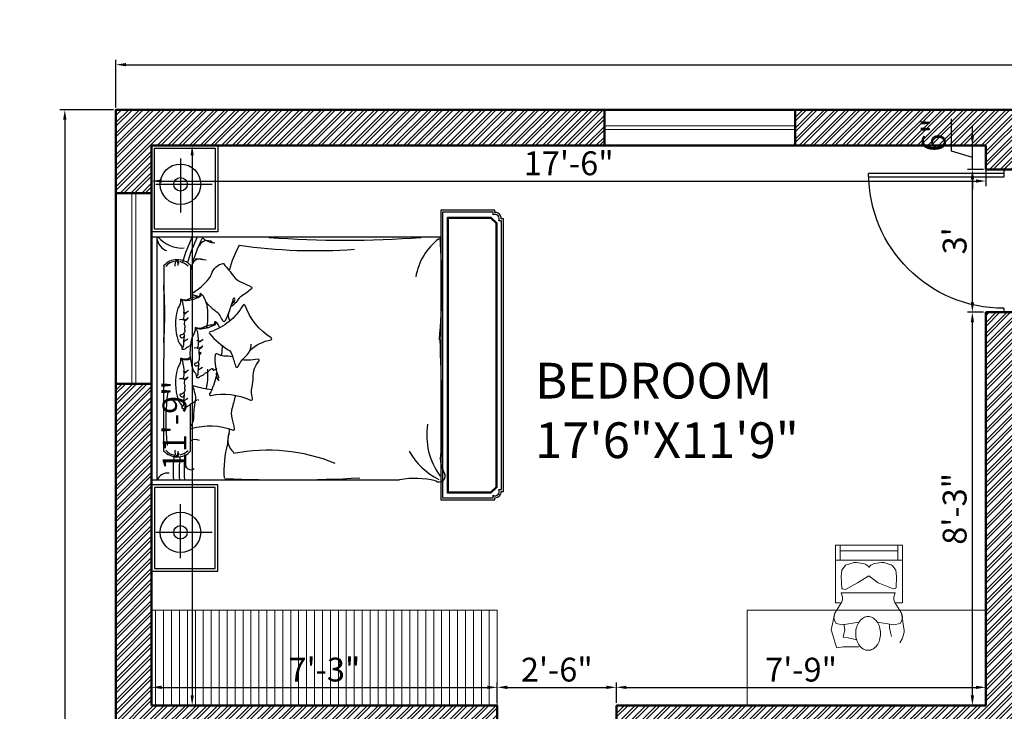
# Model space of a CAD drawing. Units: inches. Extents: x 3590 to 5167, y 65 to 1917.
# Tile 4 of 100: x 3621 to 3869, y 438 to 612. Entities that reach past the tile are written whole.
import ezdxf

# ---------------------------------------------------------------- set-up
doc = ezdxf.new("R2010")
doc.units = ezdxf.units.IN
for name, color, linetype, lineweight in [('A-ANNO-DIMS', 2, 'Continuous', 18), ('A-AREA-IDEN', 7, 'Continuous', 18), ('A-DOOR', 3, 'Continuous', 25), ('A-FURN', 21, 'Continuous', 18), ('A-GLAZ', 4, 'Continuous', 18), ('A-WALL', 7, 'Continuous', 50), ('A-WALL-PATT', 251, 'Continuous', 13)]:
    doc.layers.add(name, color=color, linetype=linetype, lineweight=lineweight)
for name, color, linetype in [('FUR', 42, 'Continuous'), ('HA-FUR', 8, 'Continuous'), ('HA-P', 8, 'Continuous'), ('SAN', 5, 'Continuous'), ('wood', 26, 'Continuous')]:
    doc.layers.add(name, color=color, linetype=linetype)
doc.styles.get("Standard").update_dxf_attribs({"font": 'arial.ttf'})
doc.dimstyles.new('ISO-25', dxfattribs={"dimtxt": 9, "dimasz": 2.5, "dimexe": 1.25, "dimexo": 0.625, "dimtad": 1, "dimdec": 1, "dimlunit": 3, "dimtxsty": 'Standard', "dimcen": 2.5, "dimadec": 0, "dimazin": 0, "dimtfac": 1, "dimtdec": 1, "dimtmove": 0, "dimatfit": 3, "dimfxl": 1, "dimarcsym": 0})

# ---------------------------------------------------------------- blocks, each defined once
blk = doc.blocks.new('*D247')
at = {"layer": 'A-ANNO-DIMS', "color": 0, "lineweight": -2, "transparency": 16777216}
for p, q in [((3645.51, 589.68), (3645.51, 601.68)), ((3648.01, 600.43), (4303.01, 600.43)), ((4305.51, 589.68), (4305.51, 601.68))]:
    blk.add_line(p, q, dxfattribs=at)
at = {"layer": 'A-ANNO-DIMS', "color": 0, "transparency": 16777216}
for points in [[(3648.01, 600.84), (3648.01, 600.01), (3645.51, 600.43)], [(4303.01, 600.84), (4303.01, 600.01), (4305.51, 600.43)]]:
    blk.add_solid(points, dxfattribs=at)
at = {"layer": 'Defpoints', "color": 0, "transparency": 16777216}
for p in [(4305.51, 600.43), (3645.51, 589.06), (4305.51, 589.06)]:
    blk.add_point(p, dxfattribs=at)
at = {"layer": 'A-ANNO-DIMS', "color": 0, "transparency": 16777216, "insert": (3975.51, 605.63), "char_height": 9, "attachment_point": 5}
blk.add_mtext("55'", dxfattribs=at)
blk = doc.blocks.new('*D248')
at = {"layer": 'A-ANNO-DIMS', "color": 0, "lineweight": -2, "transparency": 16777216}
for p, q in [((3644.89, 589.06), (3631.39, 589.06)), ((3632.64, 586.56), (3632.64, 111.56)), ((3644.89, 109.06), (3631.39, 109.06))]:
    blk.add_line(p, q, dxfattribs=at)
at = {"layer": 'A-ANNO-DIMS', "color": 0, "transparency": 16777216}
for points in [[(3632.22, 586.56), (3633.06, 586.56), (3632.64, 589.06)], [(3632.22, 111.56), (3633.06, 111.56), (3632.64, 109.06)]]:
    blk.add_solid(points, dxfattribs=at)
at = {"layer": 'Defpoints', "color": 0, "transparency": 16777216}
for p in [(3645.51, 589.06), (3632.64, 109.06), (3645.51, 109.06)]:
    blk.add_point(p, dxfattribs=at)
at = {"layer": 'A-ANNO-DIMS', "color": 0, "transparency": 16777216, "insert": (3627.42, 349.06), "char_height": 9, "attachment_point": 5, "rotation": 90}
blk.add_mtext("40'", dxfattribs=at)
blk = doc.blocks.new('D1')
for p, q in [((1, 0), (1, 34)), ((2, 0), (2, 33.99)), ((0, 0), (2, 0)), ((35, 0), (36, 0))]:
    blk.add_line(p, q)
at = {"ltscale": 0.5}
blk.add_arc((1, 0), 34, 0, 90, dxfattribs=at)
blk = doc.blocks.new('*D191')
at = {"layer": 'A-ANNO-DIMS', "color": 0, "lineweight": -2, "transparency": 16777216}
for p, q in [((3654.51, 579.43), (3654.51, 569.87)), ((3864.51, 579.43), (3864.51, 569.87)), ((3657.01, 571.12), (3862.01, 571.12))]:
    blk.add_line(p, q, dxfattribs=at)
at = {"layer": 'A-ANNO-DIMS', "color": 0, "transparency": 16777216}
for points in [[(3657.01, 571.54), (3657.01, 570.71), (3654.51, 571.12)], [(3862.01, 571.54), (3862.01, 570.71), (3864.51, 571.12)]]:
    blk.add_solid(points, dxfattribs=at)
at = {"layer": 'Defpoints', "color": 0, "transparency": 16777216}
for p in [(3654.51, 580.06), (3864.51, 580.06), (3864.51, 571.12)]:
    blk.add_point(p, dxfattribs=at)
at = {"layer": 'A-ANNO-DIMS', "color": 0, "transparency": 16777216, "insert": (3759.51, 574.81), "char_height": 6, "attachment_point": 5}
blk.add_mtext('17\'-6"', dxfattribs=at)
blk = doc.blocks.new('*D192')
at = {"layer": 'A-ANNO-DIMS', "color": 0, "lineweight": -2, "transparency": 16777216}
for p, q in [((3655.14, 580.06), (3665.95, 580.06)), ((3664.7, 577.56), (3664.7, 441.56)), ((3655.14, 439.06), (3665.95, 439.06))]:
    blk.add_line(p, q, dxfattribs=at)
at = {"layer": 'A-ANNO-DIMS', "color": 0, "transparency": 16777216}
for points in [[(3664.29, 577.56), (3665.12, 577.56), (3664.7, 580.06)], [(3664.29, 441.56), (3665.12, 441.56), (3664.7, 439.06)]]:
    blk.add_solid(points, dxfattribs=at)
at = {"layer": 'Defpoints', "color": 0, "transparency": 16777216}
for p in [(3654.51, 580.06), (3654.51, 439.06), (3664.7, 439.06)]:
    blk.add_point(p, dxfattribs=at)
at = {"layer": 'A-ANNO-DIMS', "color": 0, "transparency": 16777216, "insert": (3661.02, 509.56), "char_height": 6, "attachment_point": 5, "rotation": 90}
blk.add_mtext('11\'-9"', dxfattribs=at)
blk = doc.blocks.new('*D193')
at = {"layer": 'A-ANNO-DIMS', "color": 0, "lineweight": -2, "transparency": 16777216}
for p, q in [((3654.51, 439.68), (3654.51, 444.85)), ((3741.51, 439.68), (3741.51, 444.85)), ((3657.01, 443.6), (3739.01, 443.6))]:
    blk.add_line(p, q, dxfattribs=at)
at = {"layer": 'A-ANNO-DIMS', "color": 0, "transparency": 16777216}
for points in [[(3657.01, 444.01), (3657.01, 443.18), (3654.51, 443.6)], [(3739.01, 444.01), (3739.01, 443.18), (3741.51, 443.6)]]:
    blk.add_solid(points, dxfattribs=at)
at = {"layer": 'Defpoints', "color": 0, "transparency": 16777216}
for p in [(3741.51, 443.6), (3654.51, 439.06), (3741.51, 439.06)]:
    blk.add_point(p, dxfattribs=at)
at = {"layer": 'A-ANNO-DIMS', "color": 0, "transparency": 16777216, "insert": (3698.01, 447.29), "char_height": 6, "attachment_point": 5}
blk.add_mtext('7\'-3"', dxfattribs=at)
blk = doc.blocks.new('*D199')
at = {"layer": 'A-ANNO-DIMS', "color": 0, "lineweight": -2, "transparency": 16777216}
for p, q in [((3741.51, 439.68), (3741.51, 444.85)), ((3771.51, 439.68), (3771.51, 444.85)), ((3744.01, 443.6), (3769.01, 443.6))]:
    blk.add_line(p, q, dxfattribs=at)
at = {"layer": 'A-ANNO-DIMS', "color": 0, "transparency": 16777216}
for points in [[(3744.01, 444.01), (3744.01, 443.18), (3741.51, 443.6)], [(3769.01, 444.01), (3769.01, 443.18), (3771.51, 443.6)]]:
    blk.add_solid(points, dxfattribs=at)
at = {"layer": 'Defpoints', "color": 0, "transparency": 16777216}
for p in [(3771.51, 443.6), (3741.51, 439.06), (3771.51, 439.06)]:
    blk.add_point(p, dxfattribs=at)
at = {"layer": 'A-ANNO-DIMS', "color": 0, "transparency": 16777216, "insert": (3756.51, 447.28), "char_height": 6, "attachment_point": 5}
blk.add_mtext('2\'-6"', dxfattribs=at)
blk = doc.blocks.new('*D200')
at = {"layer": 'A-ANNO-DIMS', "color": 0, "lineweight": -2, "transparency": 16777216}
for p, q in [((3771.51, 439.68), (3771.51, 444.85)), ((3864.51, 439.68), (3864.51, 444.85)), ((3774.01, 443.6), (3862.01, 443.6))]:
    blk.add_line(p, q, dxfattribs=at)
at = {"layer": 'A-ANNO-DIMS', "color": 0, "transparency": 16777216}
for points in [[(3774.01, 444.01), (3774.01, 443.18), (3771.51, 443.6)], [(3862.01, 444.01), (3862.01, 443.18), (3864.51, 443.6)]]:
    blk.add_solid(points, dxfattribs=at)
at = {"layer": 'Defpoints', "color": 0, "transparency": 16777216}
for p in [(3864.51, 443.6), (3771.51, 439.06), (3864.51, 439.06)]:
    blk.add_point(p, dxfattribs=at)
at = {"layer": 'A-ANNO-DIMS', "color": 0, "transparency": 16777216, "insert": (3818.01, 447.28), "char_height": 6, "attachment_point": 5}
blk.add_mtext('7\'-9"', dxfattribs=at)
blk = doc.blocks.new('*D201')
at = {"layer": 'A-ANNO-DIMS', "color": 0, "lineweight": -2, "transparency": 16777216}
for p, q in [((3863.89, 538.06), (3859.88, 538.06)), ((3861.13, 441.56), (3861.13, 535.56)), ((3863.89, 439.06), (3859.88, 439.06))]:
    blk.add_line(p, q, dxfattribs=at)
at = {"layer": 'A-ANNO-DIMS', "color": 0, "transparency": 16777216}
for points in [[(3860.71, 535.56), (3861.55, 535.56), (3861.13, 538.06)], [(3860.71, 441.56), (3861.55, 441.56), (3861.13, 439.06)]]:
    blk.add_solid(points, dxfattribs=at)
at = {"layer": 'Defpoints', "color": 0, "transparency": 16777216}
for p in [(3861.13, 538.06), (3864.51, 538.06), (3864.51, 439.06)]:
    blk.add_point(p, dxfattribs=at)
at = {"layer": 'A-ANNO-DIMS', "color": 0, "transparency": 16777216, "insert": (3857.44, 488.56), "char_height": 6, "attachment_point": 5, "rotation": 90}
blk.add_mtext('8\'-3"', dxfattribs=at)
blk = doc.blocks.new('*D202')
at = {"layer": 'A-ANNO-DIMS', "color": 0, "lineweight": -2, "transparency": 16777216}
for p, q in [((3863.89, 574.06), (3859.88, 574.06)), ((3861.13, 540.56), (3861.13, 571.56)), ((3863.89, 538.06), (3859.88, 538.06))]:
    blk.add_line(p, q, dxfattribs=at)
at = {"layer": 'A-ANNO-DIMS', "color": 0, "transparency": 16777216}
for points in [[(3860.71, 571.56), (3861.55, 571.56), (3861.13, 574.06)], [(3860.71, 540.56), (3861.55, 540.56), (3861.13, 538.06)]]:
    blk.add_solid(points, dxfattribs=at)
at = {"layer": 'Defpoints', "color": 0, "transparency": 16777216}
for p in [(3861.13, 574.06), (3864.51, 574.06), (3864.51, 538.06)]:
    blk.add_point(p, dxfattribs=at)
at = {"layer": 'A-ANNO-DIMS', "color": 0, "transparency": 16777216, "insert": (3857.44, 556.06), "char_height": 6, "attachment_point": 5, "rotation": 90}
blk.add_mtext("3'", dxfattribs=at)
blk = doc.blocks.new('*D165')
at = {"layer": 'A-ANNO-DIMS', "color": 0, "lineweight": -2, "transparency": 16777216}
for p, q in [((3855.88, 578.64), (3855.88, 586.81)), ((3861.13, 582.56), (3861.13, 585.06)), ((3863.89, 580.06), (3859.88, 580.06)), ((3861.13, 574.06), (3861.13, 580.06)), ((3861.13, 574.06), (3861.13, 580.06)), ((3861.13, 577.06), (3855.88, 578.64)), ((3863.89, 574.06), (3859.88, 574.06)), ((3861.13, 571.56), (3861.13, 569.06))]:
    blk.add_line(p, q, dxfattribs=at)
at = {"layer": 'A-ANNO-DIMS', "color": 0, "transparency": 16777216}
for points in [[(3860.71, 582.56), (3861.55, 582.56), (3861.13, 580.06)], [(3860.71, 571.56), (3861.55, 571.56), (3861.13, 574.06)]]:
    blk.add_solid(points, dxfattribs=at)
at = {"layer": 'Defpoints', "color": 0, "transparency": 16777216}
for p in [(3861.13, 580.06), (3864.51, 580.06), (3864.51, 574.06)]:
    blk.add_point(p, dxfattribs=at)
at = {"layer": 'A-ANNO-DIMS', "color": 0, "transparency": 16777216, "insert": (3852.19, 582.72), "char_height": 6, "attachment_point": 5, "rotation": 90}
blk.add_mtext('6"', dxfattribs=at)
blk = doc.blocks.new('A$C0A42580C')
at = {"layer": 'SAN'}
for p, q in [((0.2873, 0.0301), (0.2873, 0.4484)), ((2.8678, 0.0301), (2.8678, 0.4484)), ((0.0949, 0.2135), (0.4958, 0.2135)), ((3.0601, 0.2135), (2.6592, 0.2135))]:
    blk.add_line(p, q, dxfattribs=at)
for centre, radius in [((0.2873, 0.2135), 0.15), ((2.8678, 0.2135), 0.15), ((0.2873, 0.2135), 0.05), ((2.8678, 0.2135), 0.05)]:
    blk.add_circle(centre, radius, dxfattribs=at)
at = {"layer": 'wood'}
for p, q in [((0.6775, 0.8851), (0.6775, 2.1392)), ((2.4775, 0.8016), (2.4775, 1.838)), ((2.4775, 0), (2.4775, 0.8016)), ((1.6633, 0.3438), (1.6434, 0.3761)), ((1.5, 0.3423), (1.5016, 0.3142)), ((0.888, 0.289), (1.1327, 0.289)), ((1.2906, 0.2348), (1.2921, 0.2067)), ((1.4538, 0.2362), (1.434, 0.2685)), ((1.7287, 0.2348), (1.7302, 0.2067)), ((1.8919, 0.2362), (1.8721, 0.2685)), ((2.267, 0.289), (1.9163, 0.289)), ((0.8909, 0.089), (1.5775, 0.089)), ((2.2642, 0.089), (1.5775, 0.089)), ((0.6775, 0.039), (2.4775, 0.039)), ((0.6775, 0), (2.4775, 0))]:
    blk.add_line(p, q, dxfattribs=at)
blk.add_lwpolyline([(0.6775, 0), (0.6775, 0.8851)], dxfattribs=at)
for points in [[(1.516, 0.7294, -0.128392), (1.4401, 0.8834, 0.70791), (1.427, 0.8863, -0.16964), (1.1848, 0.6919, 0.664036), (1.184, 0.6776, -0.184649), (1.3819, 0.4332, 0.662242), (1.3969, 0.4309, 0.078539), (1.5137, 0.5669, -0.1736), (1.5484, 0.5947, -0.02159), (1.6357, 0.6205, 0.697276), (1.6379, 0.6405, -0.093019), (1.5606, 0.699, 0.216632), (1.4719, 0.7371, -2.511293)], [(1.1211, 0.3454, 0.032543), (1.1095, 0.3091, -0.658965), (1.0917, 0.3063, 0.074753), (0.9887, 0.4234, 0.100988), (0.953, 0.4429, -0.270711), (0.8753, 0.5273, -0.276825), (0.8775, 0.5337, -0.014937), (0.9701, 0.6081, 0.134834), (1.0135, 0.6643, -0.023706), (1.0474, 0.7372, -0.664036), (1.0616, 0.7394, -0.035987), (1.119, 0.6627, 0.118631), (1.1415, 0.6412, -0.132738), (1.1955, 0.5864)], [(1.6795, 0.4818, 0.263265), (1.7191, 0.4839, -0.026108), (1.743, 0.4973, 0.027613), (1.7137, 0.4764, -0.089259), (1.8403, 0.429, 0.662242), (1.8528, 0.4376, -0.162037), (1.8882, 0.732, 0.676499), (1.8733, 0.748, -0.160513), (1.7901, 0.7439, 0.07473), (1.7202, 0.7523, -0.187721), (1.5966, 0.7963, 0.70791), (1.5851, 0.7895, -0.010003), (1.5921, 0.7143, -0.07079), (1.5891, 0.6719, 0.099539)], [(1.1759, 0.5928, 0.013884), (1.1549, 0.6131, 0.174178), (1.1437, 0.6177, 0.104076), (1.1358, 0.6165, 0.389829), (1.1324, 0.6097, 0.296089), (1.1415, 0.6019, -0.036701), (1.1572, 0.5985, -0.040547), (1.3022, 0.543, -0.70791), (1.3021, 0.5296, -0.016811), (1.2631, 0.5085, 0.11866), (1.2414, 0.4904, -0.048791), (1.1649, 0.4055, 0.103757)], [(1.5674, 0.601, 0.057807), (1.5606, 0.5339, -0.173425), (1.5457, 0.49, 0.589988), (1.5538, 0.4706, 0.137312), (1.7236, 0.4985, 0.137312)], [(1.8113, 0.4446, -0.069098), (1.7831, 0.3187, 0.658965), (1.7961, 0.3062, -0.049789), (1.8516, 0.3234, -0.103757), (1.8905, 0.3233, 0.055725), (2.0203, 0.3103, -0.11866), (2.0478, 0.304, 0.016811), (2.0881, 0.2856, 0.70791), (2.0989, 0.2936, -0.16964), (2.1104, 0.604, 0.664036), (2.1001, 0.6139, 0.023706), (2.0214, 0.597, -0.134834), (1.9505, 0.5976, 0.012748), (1.8522, 0.6228)], [(1.3107, 0.4764, 0.145733), (1.3069, 0.4677, 0.488583), (1.3089, 0.4657, -0.012138), (1.3131, 0.4661, -0.125673), (1.3213, 0.4646, -0.750706)], [(1.3153, 0.4751, -0.274893), (1.3379, 0.4529, 0.051436), (1.3468, 0.4293, -0.086628), (1.3532, 0.4078, 0.040196), (1.3593, 0.3772, -0.184744), (1.3556, 0.3344, -2.554464)], [(1.317, 0.4683, -0.060098), (1.3283, 0.4571, -0.16247), (1.3313, 0.4487, 0.120018), (1.3493, 0.3815, -0.060072), (1.3541, 0.3695, -0.13107), (1.3541, 0.3395, -0.024415), (1.3534, 0.3373, 0.070398), (1.3503, 0.3233, 0.528689), (1.3524, 0.3216, -0.069388), (1.3557, 0.3222, -0.158233), (1.4075, 0.3065, 0.085461), (1.4255, 0.2981, 0.147196), (1.6571, 0.3041, 0.10985), (1.6823, 0.3191, -0.179095), (1.7126, 0.3319, -2.318897)], [(1.1013, 0.3688, 0.145733), (1.0975, 0.3601, 0.488583), (1.0995, 0.3581, -0.012138), (1.1036, 0.3585, -0.125673), (1.1119, 0.357, -0.750706)], [(1.1059, 0.3675, -0.274893), (1.1285, 0.3453, 0.051436), (1.1373, 0.3217, -0.086628), (1.1438, 0.3003, 0.040196), (1.1499, 0.2696, -0.184744), (1.1462, 0.2269, -2.554464)], [(1.4359, 0.3803, -0.198519), (1.452, 0.3494, 0.826402), (1.4558, 0.349, 0.095956), (1.4561, 0.3528, 0.242899), (1.4461, 0.3686, -17.523452)], [(1.5447, 0.3525, -0.083557), (1.507, 0.3546, 0.203162), (1.4851, 0.3792, -0.208037), (1.5043, 0.3409, 0.124669), (1.4432, 0.3469, 0.965934)], [(1.5394, 0.3688, 0.145733), (1.5356, 0.3601, 0.488583), (1.5376, 0.3581, -0.012138), (1.5418, 0.3585, -0.125673), (1.55, 0.357, -0.750706)], [(1.1076, 0.3607, -0.060098), (1.1189, 0.3495, -0.16247), (1.1219, 0.3411, 0.120018), (1.1399, 0.2739, -0.060072), (1.1447, 0.2619, -0.13107), (1.1447, 0.2319, -0.024415), (1.144, 0.2297, 0.070398), (1.1409, 0.2157, 0.528689), (1.143, 0.2141, -0.069388), (1.1463, 0.2146, -0.158233), (1.1981, 0.1989, 0.085461), (1.2161, 0.1905, 0.147196), (1.4477, 0.1965, 0.10985), (1.4728, 0.2115, -0.179095), (1.5032, 0.2244, -2.318897)], [(1.3509, 0.3219, -0.117141), (1.3688, 0.335, -0.025084), (1.4533, 0.348, 0.033691)], [(1.5447, 0.3525, -0.008229), (1.5728, 0.3519, 0.033691)], [(1.5728, 0.3519, -0.46905), (1.6152, 0.321, 0.420988), (1.62, 0.3169, 0.857652), (1.6221, 0.3484, 0.548526)], [(1.603, 0.3451, -0.099719), (1.6221, 0.3484, 0.102691)], [(1.6214, 0.3487, -0.010168), (1.6558, 0.3447, 0.033691), (1.6907, 0.3423, -0.220869), (1.7148, 0.3311, -0.288972)], [(1.1415, 0.2143, -0.117141), (1.1594, 0.2274, -0.025084), (1.2439, 0.2405, 0.033691)], [(1.2265, 0.2728, -0.198519), (1.2426, 0.2418, 0.826402), (1.2463, 0.2415, 0.095956), (1.2467, 0.2452, 0.242899), (1.2366, 0.2611, -17.523452)], [(1.3353, 0.2449, -0.083557), (1.2976, 0.247, 0.203162), (1.2757, 0.2717, -0.208037), (1.2948, 0.2333, 0.124669), (1.2338, 0.2393, 0.965934)], [(1.3353, 0.2449, -0.008229), (1.3633, 0.2443, 0.033691)], [(1.3633, 0.2443, -0.46905), (1.4058, 0.2134, 0.420988), (1.4106, 0.2093, 0.857652), (1.4127, 0.2408, 0.548526)], [(1.3936, 0.2375, -0.099719), (1.4127, 0.2408, 0.102691)], [(1.412, 0.2411, -0.010168), (1.4464, 0.2371, 0.033691), (1.4812, 0.2348, -0.220869), (1.5054, 0.2235, -0.288972)], [(1.5721, 0.286, 0.022869), (1.578, 0.2739, -0.060072), (1.5828, 0.2619, -0.13107), (1.5828, 0.2319, -0.024415), (1.5821, 0.2297, 0.070398), (1.579, 0.2157, 0.528689), (1.5811, 0.2141, -0.069388), (1.5844, 0.2146, -0.158233), (1.6362, 0.1989, 0.085461), (1.6542, 0.1905, 0.147196), (1.8858, 0.1965, 0.10985), (1.911, 0.2115, -0.179095), (1.9413, 0.2244, -2.318897)], [(1.5796, 0.2143, -0.117141), (1.5975, 0.2274, -0.025084), (1.682, 0.2405, 0.033691)], [(1.5838, 0.2873, 0.023398), (1.588, 0.2696, -0.184744), (1.5843, 0.2269, -2.554464)], [(1.6646, 0.2728, -0.198519), (1.6807, 0.2418, 0.826402), (1.6845, 0.2415, 0.095956), (1.6848, 0.2452, 0.242899), (1.6748, 0.2611, -17.523452)], [(1.7734, 0.2449, -0.083557), (1.7357, 0.247, 0.203162), (1.7138, 0.2717, -0.208037), (1.733, 0.2333, 0.124669), (1.6719, 0.2393, 0.965934)], [(1.7734, 0.2449, -0.008229), (1.8015, 0.2443, 0.033691)], [(1.8015, 0.2443, -0.46905), (1.8439, 0.2134, 0.420988), (1.8487, 0.2093, 0.857652), (1.8508, 0.2408, 0.548526)], [(1.8317, 0.2375, -0.099719), (1.8508, 0.2408, 0.102691)], [(1.8501, 0.2411, -0.010168), (1.8845, 0.2371, 0.033691), (1.9193, 0.2348, -0.220869), (1.9435, 0.2235, -0.288972)]]:
    blk.add_lwpolyline(points, format="xyb", dxfattribs=at)
for points in [[(0.64, 0), (0, 0), (0, 0.49), (0.64, 0.49)], [(0.62, 0.02), (0.02, 0.02), (0.02, 0.47), (0.62, 0.47)], [(2.515, 0), (3.155, 0), (3.155, 0.49), (2.515, 0.49)], [(2.535, 0.02), (3.135, 0.02), (3.135, 0.47), (2.535, 0.47)]]:
    blk.add_lwpolyline(points, close=True, dxfattribs=at)
for centre, radius, start, end in [((1.0344, -2.14), 4.292, 84.56078, 94.7164), ((1.0494, 2.4026), 0.4515, 217.47941, 260.35986), ((2.0208, -11.0786), 13.2288, 88.75549, 92.51133), ((2.1491, 2.5471), 0.5083, 260.65485, 306.44155), ((2.3125, 2.3833), 0.2443, 254.1515, 300.95574), ((2.0168, 2.3573), 0.5127, 299.08175, 333.44367), ((2.4501, 2.1309), 0.0445, 324.18954, 118.92203), ((3.1371, 1.9502), 0.669, 166.6404, 189.65708), ((-7.0839, 1.4328), 7.7858, 355.84817, 4.15183), ((-7.2439, 0.9937), 9.7233, 357.34474, 3.23068), ((-3.167, 1.2143), 3.9465, 351.77286, 4.18386), ((3.5803, 0.8622), 1.3213, 157.81295, 191.15154), ((1.1611, 1.4181), 0.8768, 241.21362, 254.41879), ((2.181, 0.6859), 0.1221, 247.37754, 321.13165), ((1.2583, 0.6364), 0.0695, 238.58923, 301.92671), ((1.4714, 0.0722), 0.4528, 80.62397, 88.74059), ((1.4035, -0.3388), 0.8693, 79.71489, 80.62397), ((1.7861, -2.1601), 2.7557, 80.89877, 83.46656), ((2.4192, 1.3819), 0.8461, 255.77539, 273.25587), ((0.5904, 0.4689), 0.13, 317.38218, 359.70393), ((0.7723, 0.4131), 0.0674, 147.68233, 245.79865), ((1.3546, 0.4469), 0.0529, 114.21284, 146.15395), ((2.6126, -2.3504), 3.1201, 113.83178, 114.21284), ((1.6301, 0.4539), 0.0342, 31.14095, 54.95422), ((1.6709, 0.4489), 0.0156, 131.9623, 212.08127), ((1.6729, 0.4422), 0.0178, 140.41793, 157.63267), ((1.7235, 0.4818), 0.0777, 212.08127, 227.364), ((1.6635, 0.4499), 0.00568, 95.52245, 140.41793), ((1.5664, 0.4154), 0.1086, 24.20989, 31.14095), ((1.6627, 0.4587), 0.00309, 275.52245, 24.20989), ((1.1611, 1.3191), 1.0568, 242.76671, 257.10398), ((0.0312, 0.4583), 0.8174, 350.42368, 356.2506), ((0.9021, 0.3562), 0.0605, 155.8342, 254.41058), ((1.1452, 0.3394), 0.0529, 114.21284, 146.15395), ((2.4032, -2.458), 3.1201, 113.55686, 114.21284), ((1.2046, 0.2912), 0.121, 99.42032, 113.55686), ((1.2774, -0.1478), 0.5659, 95.90379, 99.42032), ((1.2626, -0.005), 0.4223, 88.74059, 95.90379), ((1.2619, -0.0354), 0.4528, 80.62397, 88.74059), ((1.1941, -0.4464), 0.8693, 79.45871, 80.62397), ((1.4207, 0.3463), 0.0342, 31.14095, 54.95422), ((1.7007, -0.005), 0.4223, 88.74059, 95.90379), ((1.6391, 0.3902), 0.0469, 17.32618, 47.364), ((1.7106, 0.4125), 0.028, 197.32618, 226.17302), ((1.6431, 0.3422), 0.0695, 26.61764, 46.17302), ((1.8202, 0.431), 0.1287, 206.61764, 215.96192), ((1.7001, -0.0354), 0.4528, 80.62397, 88.74059), ((1.6322, -0.4464), 0.8693, 78.43923, 80.62397), ((1.1611, 1.3191), 1.0937, 243.75553, 254.4906), ((1.1611, 1.2816), 1.0937, 243.75553, 254.38927), ((1.4614, 0.3413), 0.0156, 131.9623, 212.08127), ((1.4635, 0.3347), 0.0178, 140.41793, 157.63267), ((1.4541, 0.3424), 0.00568, 95.52245, 140.41793), ((1.357, 0.3078), 0.1086, 24.20989, 31.14095), ((1.4533, 0.3511), 0.00309, 275.52245, 24.20989), ((1.5012, 0.305), 0.028, 197.32618, 226.17302), ((1.715, 0.3349), 0.00379, 207.1817, 328.02977), ((1.6975, 0.3419), 0.023, 350.76434, 35.96192), ((1.7058, 0.3406), 0.0145, 328.02977, 350.76434), ((1.9016, 0.3347), 0.0178, 140.41793, 157.63267), ((1.9522, 0.3743), 0.0777, 212.08127, 227.364), ((1.8922, 0.3424), 0.00568, 95.52245, 140.41793), ((1.8678, 0.2827), 0.0469, 17.32618, 47.364), ((1.9393, 0.305), 0.028, 197.32618, 226.17302), ((2.2511, 0.3256), 0.071, 155.86842, 211.04513), ((2.3616, 0.2915), 0.0419, 290.78583, 35.36309), ((0.5293, 0.2241), 0.2307, 309.63048, 4.27465), ((0.9846, 0.1903), 0.1381, 134.39284, 227.23745), ((0.9986, 0.1735), 0.1427, 136.58239, 164.9725), ((1.4337, 0.2347), 0.0695, 26.61764, 46.17302), ((1.6108, 0.3235), 0.1287, 206.61764, 215.96192), ((1.5055, 0.2273), 0.00379, 207.1817, 328.02977), ((1.4881, 0.2344), 0.023, 350.76434, 35.96192), ((1.4964, 0.233), 0.0145, 328.02977, 350.76434), ((1.8718, 0.2347), 0.0695, 26.61764, 46.17302), ((2.0489, 0.3235), 0.1287, 206.61764, 215.96192), ((1.9436, 0.2273), 0.00379, 207.1817, 328.02977), ((1.9262, 0.2344), 0.023, 350.76434, 35.96192), ((1.9345, 0.233), 0.0145, 328.02977, 350.76434), ((2.1565, 0.1735), 0.1427, 15.0275, 43.41761), ((2.1704, 0.1903), 0.1381, 312.76255, 45.60716), ((2.4192, 1.2667), 1.0261, 263.09035, 273.25587), ((0.8396, 0.185), 0.0112, 314.89662, 45.10338), ((0.8413, 0.1846), 0.0128, 299.47062, 57.44416), ((0.8844, 0.2286), 0.0569, 229.70587, 281.11527), ((0.8802, 0.1371), 0.0592, 81.47786, 123.11925), ((0.8698, 0.1793), 0.0229, 77.14902, 159.1786), ((0.9466, 0.1765), 0.0862, 185.53723, 234.68694), ((2.2085, 0.1765), 0.0862, 305.31306, 354.46277), ((2.2706, 0.2286), 0.0569, 258.88473, 310.29413), ((2.2749, 0.1371), 0.0592, 56.88075, 98.52214), ((2.2853, 0.1793), 0.0229, 20.8214, 102.85098), ((2.4192, 1.2218), 1.0629, 263.23622, 273.25587), ((2.3138, 0.1846), 0.0128, 122.55584, 240.52938), ((2.3154, 0.185), 0.0112, 134.89662, 225.10338), ((2.4192, 1.2667), 1.0629, 263.94374, 273.25587), ((0.6729, 0.151), 0.1135, 279.23824, 338.73819), ((1.2481, -2.5919), 2.6893, 85.4722, 94.5278), ((2.0447, 1.7022), 1.5979, 262.13639, 276.48786), ((2.508, 0.1152), 0.0792, 169.94668, 248.24015)]:
    blk.add_arc(centre, radius, start, end, dxfattribs=at)
blk = doc.blocks.new('A$C623F1DA0')
at = {"layer": 'FUR'}
blk.add_lwpolyline([(0.628, 2.912, 0.414214), (0.562, 2.978), (0.562, 3), (0, 3), (0, 0), (0.562, 0), (0.562, 0.022, 0.414214), (0.628, 0.088), (0.65, 0.088), (0.65, 2.912)], format="xyb", close=True, dxfattribs=at)
at = {"layer": 'HA-FUR'}
blk.add_lwpolyline([(0.603, 2.892, 0.710288), (0.542, 2.953), (0.542, 2.98), (0.02, 2.98), (0.02, 0.02), (0.542, 0.02), (0.542, 0.047, 0.710288), (0.603, 0.108), (0.63, 0.108), (0.63, 2.892)], format="xyb", close=True, dxfattribs=at)
at = {"layer": 'HA-P'}
for points in [[(0.07, 2.93), (0.521, 2.93), (0.58, 2.871), (0.58, 0.129), (0.521, 0.07), (0.07, 0.07)], [(0.08, 2.92), (0.517, 2.92), (0.57, 2.867), (0.57, 0.133), (0.517, 0.08), (0.08, 0.08)]]:
    blk.add_lwpolyline(points, close=True, dxfattribs=at)

msp = doc.modelspace()

# ---------------------------------------------------------------- hatches: boundary and pattern name
at = {"layer": 'A-WALL-PATT', "transparency": 33554687}
h = msp.add_hatch(dxfattribs=at)
h.set_pattern_fill('ANSI32', color=256, scale=0.2)
h.set_pattern_definition([(45, (0, -1216.9392), (-1.3470384, 1.3470384), []), (45, (0.898, -1216.9392), (-1.3470384, 1.3470384), [])])
h.paths.add_polyline_path([(3768.51, 589.06), (3645.51, 589.06), (3645.51, 568.06), (3654.51, 568.06), (3654.51, 580.06), (3671.16, 580.06), (3768.51, 580.06)])
h.paths.add_polyline_path([(3909.51, 589.06), (3816.51, 589.06), (3816.51, 580.06), (3864.51, 580.06), (3864.51, 574.06), (3873.51, 574.06), (3873.51, 580.06), (3909.51, 580.06)])
h.paths.add_polyline_path([(4053.51, 589.06), (3969.51, 589.06), (3969.51, 580.06), (4053.51, 580.06)])
h.paths.add_polyline_path([(4215.51, 589.06), (4113.51, 589.06), (4113.51, 580.06), (4206.51, 580.06), (4206.51, 574.06), (4215.51, 574.06)])
h.paths.add_polyline_path([(3654.51, 520.06), (3645.51, 520.06), (3645.51, 403.06), (3654.51, 403.06), (3654.51, 433.06), (3741.51, 433.06), (3741.51, 439.06), (3654.51, 439.06)], flags=17)
h.paths.add_polyline_path([(3873.51, 538.06), (3864.51, 538.06), (3864.51, 439.06), (3771.51, 439.06), (3771.51, 433.06), (3774.51, 433.06), (3774.51, 337.06), (3654.51, 337.06), (3654.51, 367.06), (3645.51, 367.06), (3645.51, 322.06), (3654.51, 322.06), (3654.51, 328.06), (3864.51, 328.06), (3864.51, 322.06), (3873.51, 322.06), (3873.51, 367.06), (3864.51, 367.06), (3864.51, 337.06), (3780.51, 337.06), (3780.51, 433.06), (3864.51, 433.06), (3864.51, 403.06), (3873.51, 403.06)])
h.paths.add_polyline_path([(3654.51, 274.06), (3645.51, 274.06), (3645.51, 109.06), (3810.51, 109.06), (3810.51, 118.06), (3809.96, 118.06), (3654.51, 118.06)])
h.paths.add_polyline_path([(3915.51, 118.06), (3873.51, 118.06), (3873.51, 135.93), (3873.51, 205.06), (3876.51, 205.06), (3876.51, 214.06), (3864.51, 214.06), (3864.51, 118.06), (3858.51, 118.06), (3858.51, 109.06), (3915.51, 109.06)])
h.paths.add_polyline_path([(4028.01, 118.06), (4002.51, 118.06), (4002.51, 286.06), (3981.51, 286.06), (3981.51, 277.06), (3993.51, 277.06), (3993.51, 214.06), (3921.51, 214.06), (3921.51, 277.06), (3933.51, 277.06), (3933.51, 286.06), (3864.51, 286.06), (3864.51, 277.06), (3912.51, 277.06), (3912.51, 214.06), (3906.51, 214.06), (3906.51, 205.06), (3993.51, 205.06), (3993.51, 118.06), (3951.51, 118.06), (3951.51, 109.06), (4028.01, 109.06)])
h.paths.add_polyline_path([(4203.51, 118.06), (4158.51, 118.06), (4158.51, 310.06), (4194.51, 310.06), (4194.51, 319.06), (4149.51, 319.06), (4149.51, 118.06), (4124.01, 118.06), (4124.01, 109.06), (4203.51, 109.06)])
h.paths.add_polyline_path([(4305.51, 349.06), (4296.51, 349.06), (4296.51, 319.06), (4278.64, 319.06), (4260.51, 319.06), (4260.51, 310.06), (4296.51, 310.06), (4296.51, 304.06), (4305.51, 304.06)])
h.paths.add_polyline_path([(4305.51, 256.06), (4296.51, 256.06), (4296.51, 118.06), (4251.51, 118.06), (4251.51, 109.06), (4305.51, 109.06)])
h.paths.add_polyline_path([(4305.51, 460.06), (4215.51, 460.06), (4215.51, 526.06), (4206.51, 526.06), (4206.51, 460.06), (4149.51, 460.06), (4149.51, 451.06), (4296.51, 451.06), (4296.51, 421.06), (4305.51, 421.06)])

# ---------------------------------------------------------------- linework, layer by layer
at = {"layer": 'A-FURN'}
for p, q in [((3826.65, 479.38), (3826.65, 464.87)), ((3843.5, 479.38), (3826.65, 479.38)), ((3827.81, 475.61), (3827.81, 479.38)), ((3842.4, 475.61), (3842.4, 479.38)), ((3843.5, 464.87), (3843.5, 479.38)), ((3842.4, 477.94), (3827.81, 477.94)), ((3843.5, 475.61), (3826.65, 475.61)), ((3828.27, 473.11), (3829.16, 474.36)), ((3829.16, 474.36), (3831.09, 474.95)), ((3831.91, 475.02), (3833.56, 474.82)), ((3834.86, 474.09), (3835.08, 473.82)), ((3835.29, 474.09), (3835.08, 473.82)), ((3838.24, 475.02), (3836.59, 474.82)), ((3840.35, 474.56), (3839.07, 474.95)), ((3841.88, 473.11), (3841.38, 473.82)), ((3828.09, 471.5), (3828.27, 473.11)), ((3828.26, 468.51), (3828.09, 471.5)), ((3835.08, 471.68), (3832.21, 469.88)), ((3837.4, 469.88), (3835.08, 471.68)), ((3842.06, 471.5), (3841.88, 473.11)), ((3841.9, 468.66), (3842.06, 471.5)), ((3832.21, 469.88), (3829.16, 468.27)), ((3841.17, 468.45), (3837.4, 469.88)), ((3841.83, 468.58), (3841.17, 468.45)), ((3828.09, 467.38), (3841.7, 467.38)), ((3841.7, 467.38), (3828.09, 467.38)), ((3828.09, 467.38), (3828.34, 466.63)), ((3829.16, 468.27), (3828.33, 468.44)), ((3841.7, 467.38), (3841.46, 466.63)), ((3828.16, 464.98), (3826.53, 462.27)), ((3826.65, 464.87), (3828.09, 464.87)), ((3841.64, 464.98), (3843.26, 462.27)), ((3841.7, 464.87), (3843.5, 464.87)), ((3654.51, 463.06), (3741.51, 463.06)), ((3655.51, 463.06), (3655.51, 439.06)), ((3657.51, 463.06), (3657.51, 439.06)), ((3659.51, 463.06), (3659.51, 439.06)), ((3661.51, 463.06), (3661.51, 439.06)), ((3663.51, 463.06), (3663.51, 439.06)), ((3665.51, 463.06), (3665.51, 439.06)), ((3667.51, 463.06), (3667.51, 439.06)), ((3669.51, 463.06), (3669.51, 439.06)), ((3671.51, 463.06), (3671.51, 439.06)), ((3673.51, 463.06), (3673.51, 439.06)), ((3675.51, 463.06), (3675.51, 439.06)), ((3677.51, 463.06), (3677.51, 439.06)), ((3679.51, 463.06), (3679.51, 439.06)), ((3681.51, 463.06), (3681.51, 439.06)), ((3683.51, 463.06), (3683.51, 439.06)), ((3685.51, 463.06), (3685.51, 439.06)), ((3687.51, 463.06), (3687.51, 439.06)), ((3689.51, 463.06), (3689.51, 439.06)), ((3691.51, 463.06), (3691.51, 439.06)), ((3693.51, 463.06), (3693.51, 439.06)), ((3695.51, 463.06), (3695.51, 439.06)), ((3697.51, 463.06), (3697.51, 439.06)), ((3699.51, 463.06), (3699.51, 439.06)), ((3701.51, 463.06), (3701.51, 439.06)), ((3703.51, 463.06), (3703.51, 439.06)), ((3705.51, 463.06), (3705.51, 439.06)), ((3707.51, 463.06), (3707.51, 439.06)), ((3709.51, 463.06), (3709.51, 439.06)), ((3711.51, 463.06), (3711.51, 439.06)), ((3713.51, 463.06), (3713.51, 439.06)), ((3715.51, 463.06), (3715.51, 439.06)), ((3717.51, 463.06), (3717.51, 439.06)), ((3719.51, 463.06), (3719.51, 439.06)), ((3721.51, 463.06), (3721.51, 439.06)), ((3723.51, 463.06), (3723.51, 439.06)), ((3725.51, 463.06), (3725.51, 439.06)), ((3727.51, 463.06), (3727.51, 439.06)), ((3729.51, 463.06), (3729.51, 439.06)), ((3731.51, 463.06), (3731.51, 439.06)), ((3733.51, 463.06), (3733.51, 439.06)), ((3735.51, 463.06), (3735.51, 439.06)), ((3737.51, 463.06), (3737.51, 439.06)), ((3739.51, 463.06), (3739.51, 439.06)), ((3741.51, 463.06), (3741.51, 439.06)), ((3804.47, 463.06), (3864.51, 463.06)), ((3804.47, 463.06), (3804.47, 439.06)), ((3843.26, 462.27), (3843.92, 457.92)), ((3826.5, 460.29), (3826.83, 459.68)), ((3826.83, 459.68), (3828.45, 459.32)), ((3828.45, 459.32), (3832.57, 460.04)), ((3841.35, 459.32), (3837.23, 460.04)), ((3842.96, 459.68), (3841.35, 459.32)), ((3843.3, 460.29), (3842.96, 459.68))]:
    msp.add_line(p, q, dxfattribs=at)
for points in [[(3826.53, 462.27), (3825.58, 458.07), (3826.12, 456.45), (3826.65, 454.48), (3827.01, 453.59), (3828.63, 453.77), (3830.24, 453.77), (3832.57, 453.77)], [(3832.03, 455.56), (3829.88, 456.1), (3828.63, 456.27), (3828.98, 458.07), (3828.8, 459.5)], [(3840.77, 456.44), (3840.55, 457.38), (3840.3, 458.61), (3840.3, 459.49)], [(3842.83, 454.84), (3843.48, 455.82), (3843.77, 456.8), (3843.92, 457.58), (3843.92, 458.02)]]:
    msp.add_lwpolyline(points, dxfattribs=at)
msp.add_lwpolyline([(3838.01, 457.17, 0.07405), (3837.76, 458.85, 0.084801), (3837.09, 460.17, 0.106336), (3836.03, 461.12, 0.128955), (3834.88, 461.42, 0.128955), (3833.74, 461.12, 0.106336), (3832.68, 460.17, 0.084801), (3832.01, 458.85, 0.07405), (3831.76, 457.17, 0.07405), (3832.01, 455.49, 0.084801), (3832.68, 454.17, 0.106336), (3833.74, 453.22, 0.128955), (3834.88, 452.92, 0.128955), (3836.03, 453.22, 0.106336), (3837.09, 454.17, 0.084801), (3837.76, 455.49, 0.07405)], format="xyb", close=True, dxfattribs=at)
for centre, radius, start, end in [((3831.67, 473.06), 1.98, 82.8785, 107.0946), ((3833.31, 472.85), 1.98, 38.6739, 82.8785), ((3836.84, 472.85), 1.98, 97.1215, 141.3261), ((3838.48, 473.06), 1.98, 72.9054, 97.1215), ((3839.76, 472.66), 1.98, 35.5514, 72.9054), ((3828.34, 468.52), 0.0779, 183.3682, 258.6956), ((3828.34, 468.52), 0.0779, 183.3682, 258.6956), ((3841.82, 468.66), 0.0779, 281.3044, 356.6318), ((3826.45, 466), 1.98, 329.0235, 18.4436), ((3843.34, 466), 1.98, 161.5564, 210.9765), ((3828.23, 461.25), 1.98, 149.0235, 209.0669), ((3841.56, 461.25), 1.98, 330.9331, 30.9765)]:
    msp.add_arc(centre, radius, start, end, dxfattribs=at)
at = {"layer": 'A-GLAZ'}
for p, q in [((3816.51, 585.06), (3768.51, 585.06)), ((3816.51, 584.06), (3768.51, 584.06)), ((3649.51, 520.06), (3649.51, 568.06)), ((3650.51, 520.06), (3650.51, 568.06))]:
    msp.add_line(p, q, dxfattribs=at)
at = {"layer": 'A-WALL'}
for p, q in [((3768.51, 580.06), (3768.51, 589.06)), ((3816.51, 580.06), (3816.51, 589.06)), ((3654.51, 580.06), (3864.51, 580.06)), ((3654.51, 439.06), (3654.51, 580.06)), ((3864.51, 574.06), (3864.51, 580.06)), ((3864.51, 574.06), (3873.51, 574.06)), ((3654.51, 568.06), (3645.51, 568.06)), ((3864.51, 538.06), (3873.51, 538.06)), ((3864.51, 439.06), (3864.51, 538.06)), ((3654.51, 520.06), (3645.51, 520.06)), ((3654.51, 439.06), (3741.51, 439.06)), ((3741.51, 433.06), (3741.51, 439.06)), ((3771.51, 439.06), (3864.51, 439.06)), ((3771.51, 433.06), (3771.51, 439.06))]:
    msp.add_line(p, q, dxfattribs=at)
msp.add_lwpolyline([(4305.51, 460.06), (4305.51, 109.06), (3645.51, 109.06), (3645.51, 589.06), (4215.51, 589.06)], dxfattribs=at)

# ---------------------------------------------------------------- block references
at = {"layer": 'A-DOOR', "xscale": -1, "rotation": 90}
msp.add_blockref('D1', (3869.01, 574.06), dxfattribs=at)
at = {"layer": 'A-FURN', "xscale": 33.96864568351422, "yscale": 33.96864568351422, "zscale": 33.96864568351422, "rotation": 270}
msp.add_blockref('A$C0A42580C', (3654.51, 580.06), dxfattribs=at)
at = {"layer": 'A-FURN', "xscale": 24.31060204424285, "yscale": 24.31060204424285, "zscale": 24.31060204424285}
msp.add_blockref('A$C623F1DA0', (3727.27, 490.82), dxfattribs=at)

# ---------------------------------------------------------------- texts
at = {"layer": 'A-AREA-IDEN', "insert": (3751.05, 525.34), "char_height": 9, "attachment_point": 1}
msp.add_mtext_dynamic_manual_height_columns('{\\fTimes New Roman|b0|i0|c0|p18;BEDROOM\\P17\'6"X11\'9"}', width=67.3508, gutter_width=12.5, heights=[0], dxfattribs=at)

# ---------------------------------------------------------------- dimensions: what is measured, and where the dimension line sits
at = {"layer": 'A-ANNO-DIMS'}
for base, p1, p2, override, picture, middle in [((4305.51, 600.43), (3645.51, 589.06), (4305.51, 589.06), {"dimclrd": 0, "dimclre": 0, "dimclrt": 0}, '*D247', (3975.51, 605.63)), ((3864.51, 571.12), (3654.51, 580.06), (3864.51, 580.06), {"dimtxt": 6, "dimclrd": 0, "dimclre": 0, "dimclrt": 0}, '*D191', (3759.51, 574.81)), ((3741.51, 443.6), (3654.51, 439.06), (3741.51, 439.06), {"dimtxt": 6, "dimclrd": 0, "dimclre": 0, "dimclrt": 0}, '*D193', (3698.01, 447.29)), ((3771.51, 443.6), (3741.51, 439.06), (3771.51, 439.06), {"dimtxt": 6, "dimclrd": 0, "dimclre": 0, "dimclrt": 0, "dimtmove": 1}, '*D199', (3756.51, 447.28)), ((3864.51, 443.6), (3771.51, 439.06), (3864.51, 439.06), {"dimtxt": 6, "dimclrd": 0, "dimclre": 0, "dimclrt": 0, "dimtmove": 1}, '*D200', (3818.01, 447.28))]:
    dim = msp.add_linear_dim(base=base, p1=p1, p2=p2, dimstyle='ISO-25', override=override, dxfattribs=at)
    dim.commit()
    dim.dimension.update_dxf_attribs({"geometry": picture, "text_midpoint": middle})
for base, p1, p2, override, picture, middle in [((3632.64, 109.06), (3645.51, 589.06), (3645.51, 109.06), {"dimclrd": 0, "dimclre": 0, "dimclrt": 0}, '*D248', (3627.42, 349.06)), ((3861.13, 580.06), (3864.51, 574.06), (3864.51, 580.06), {"dimtxt": 6, "dimclrd": 0, "dimclre": 0, "dimclrt": 0, "dimtmove": 1}, '*D165', (3852.19, 579.26)), ((3664.7, 439.06), (3654.51, 580.06), (3654.51, 439.06), {"dimtxt": 6, "dimclrd": 0, "dimclre": 0, "dimclrt": 0}, '*D192', (3661.02, 509.56)), ((3861.13, 574.06), (3864.51, 538.06), (3864.51, 574.06), {"dimtxt": 6, "dimclrd": 0, "dimclre": 0, "dimclrt": 0, "dimtmove": 1}, '*D202', (3857.44, 556.06)), ((3861.13, 538.06), (3864.51, 439.06), (3864.51, 538.06), {"dimtxt": 6, "dimclrd": 0, "dimclre": 0, "dimclrt": 0}, '*D201', (3857.44, 488.56))]:
    dim = msp.add_linear_dim(base=base, p1=p1, p2=p2, angle=90, dimstyle='ISO-25', override=override, dxfattribs=at)
    dim.commit()
    dim.dimension.update_dxf_attribs({"geometry": picture, "text_midpoint": middle})

doc.saveas('drawing.dxf')
